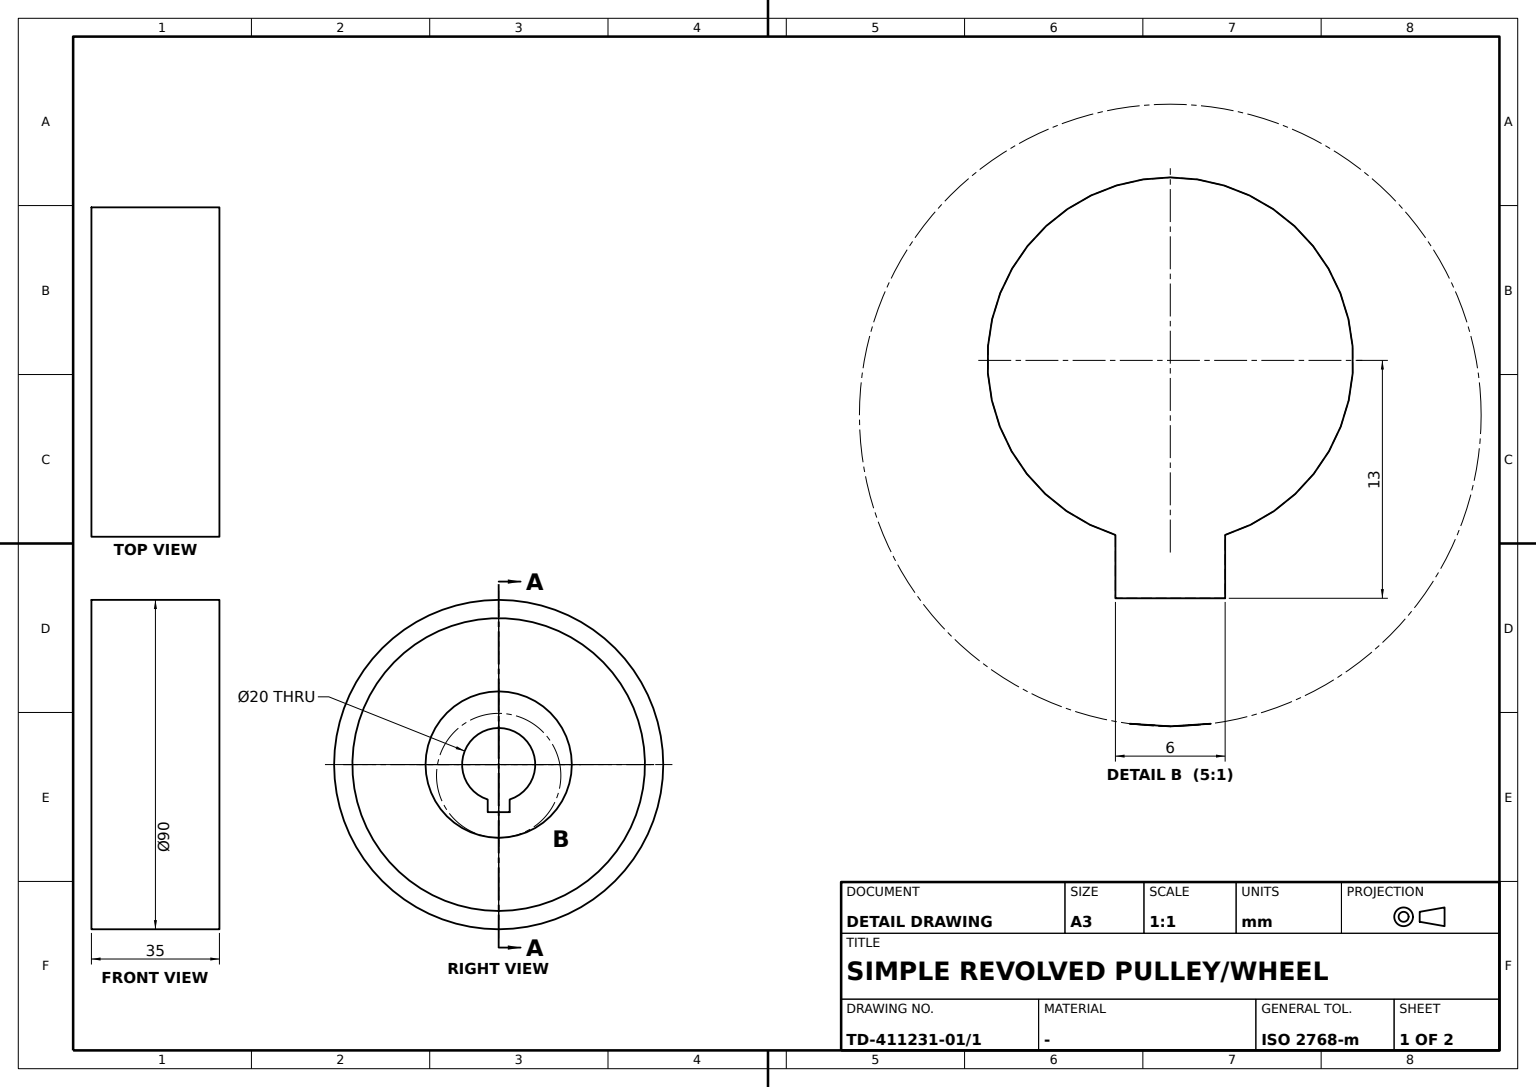
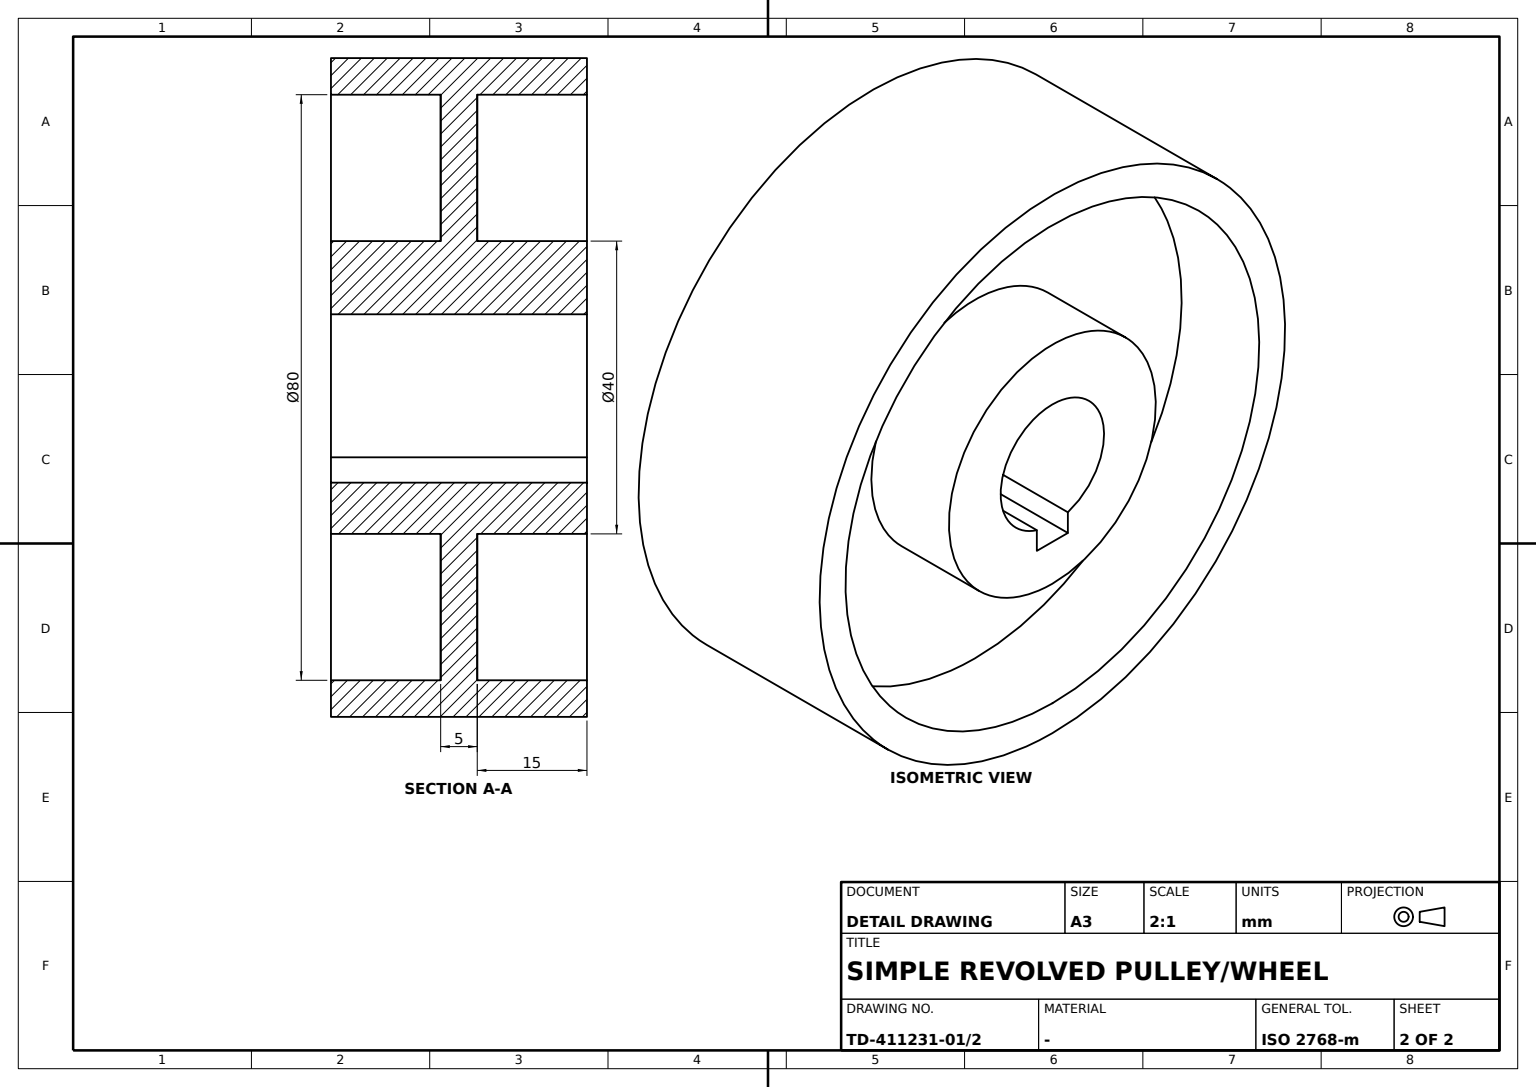
CATIA V5 part; units mm, degrees
sketch "Sketch1" plane through (0, 0, 0) normal (0, 0, 1) x (1, 0, 0)
  line L0 (0, -34.2521) -> (0, 79.5025) construction
  point P0 (0, -34.2521)
  point P1 (0, 45)
  line L1 (0, 45) -> (-17.5, 45)
  point P2 (-17.5, 45)
  line L2 (-17.5, 45) -> (-17.5, 40)
  point P3 (-17.5, 40)
  line L3 (-17.5, 40) -> (-2.5, 40)
  point P4 (-2.5, 40)
  line L4 (-2.5, 40) -> (-2.5, 20)
  point P5 (-2.5, 20)
  line L5 (-2.5, 20) -> (-17.5, 20)
  point P6 (-17.5, 20)
  line L6 (-17.5, 20) -> (-17.5, 10)
  point P7 (-17.5, 10)
  line L7 (-17.5, 10) -> (-2.5, 10)
  point P8 (-2.5, 10)
  line L8 (-2.5, 10) -> (0, 10)
  point P9 (0, 10)
  point P10 (0, 45)
  point P11 (17.5, 45)
  point P12 (17.5, 40)
  point P13 (2.5, 40)
  point P14 (2.5, 20)
  point P15 (17.5, 20)
  point P16 (17.5, 10)
  point P17 (2.5, 10)
  point P18 (0, 10)
  line L9 (0, 45) -> (17.5, 45)
  line L10 (17.5, 45) -> (17.5, 40)
  line L11 (17.5, 40) -> (2.5, 40)
  line L12 (2.5, 40) -> (2.5, 20)
  line L13 (2.5, 20) -> (17.5, 20)
  line L14 (17.5, 20) -> (17.5, 10)
  line L15 (17.5, 10) -> (2.5, 10)
  line L16 (2.5, 10) -> (0, 10)
  line L17 (-46.1932, 0) -> (102.1277, 0) construction
  point P19 (-46.1932, 0)
  dimension "distance L1 x axis" = 45
  dimension "distance L3 x axis" = 40
  dimension "distance x axis L5" = 20
  dimension "distance L7 x axis" = 10
  dimension "length L1" = 17.5
  dimension "distance L4 L0" = 2.5
  constraint coincidence P0 y-axis
  constraint coincidence P1 L0
  constraint coincidence P6 L2
  constraint coincidence P8 L4
  constraint coincidence P9 L0
  constraint coincidence P19 x-axis
  constraint coincidence P1 P10
  constraint coincidence P9 P18
  constraint vertical L0 y-axis
  constraint vertical L2 y-axis
  constraint vertical L4 y-axis
  constraint vertical L6 y-axis
  constraint horizontal L1 x-axis
  constraint horizontal L3 x-axis
  constraint horizontal L5 x-axis
  constraint horizontal L7 x-axis
  constraint horizontal L8 x-axis
  constraint horizontal L17 x-axis
  constraint symmetry P1 P10 L0
  constraint symmetry P2 P11 L0
  constraint symmetry P3 P12 L0
  constraint symmetry P4 P13 L0
  constraint symmetry P5 P14 L0
  constraint symmetry P6 P15 L0
  constraint symmetry P7 P16 L0
  constraint symmetry P8 P17 L0
  constraint symmetry P9 P18 L0
  constraint symmetry L1 L9 L0
  constraint symmetry L2 L10 L0
  constraint symmetry L3 L11 L0
  constraint symmetry L4 L12 L0
  constraint symmetry L5 L13 L0
  constraint symmetry L6 L14 L0
  constraint symmetry L7 L15 L0
  constraint symmetry L8 L16 L0
revolve "Shaft1" add sketch "Sketch1" angle 360 about L17
sketch "Sketch2" plane through (17.5, 0, 0) normal (1, 0, 0) x (0, 1, 0)
  line L0 (-3, -6.6347) -> (3, -6.6347)
  line L1 (3, -6.6347) -> (3, -13)
  line L2 (3, -13) -> (-3, -13)
  line L3 (-3, -13) -> (-3, -6.6347)
  line L4 (0, 14.5493) -> (0, -34.1909) construction
  point P0 (0, 14.5493)
  dimension "distance x axis L2" = 13
  dimension "distance L3 L1" = 6
  constraint horizontal L0 x-axis
  constraint horizontal L2 x-axis
  constraint vertical L1 y-axis
  constraint vertical L3 y-axis
  constraint vertical L4 y-axis
  constraint coincidence P0 y-axis
  constraint symmetry L3 L1 L4
extrude "Pocket1" cut sketch "Sketch2" against normal through all
